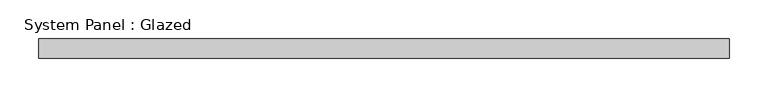
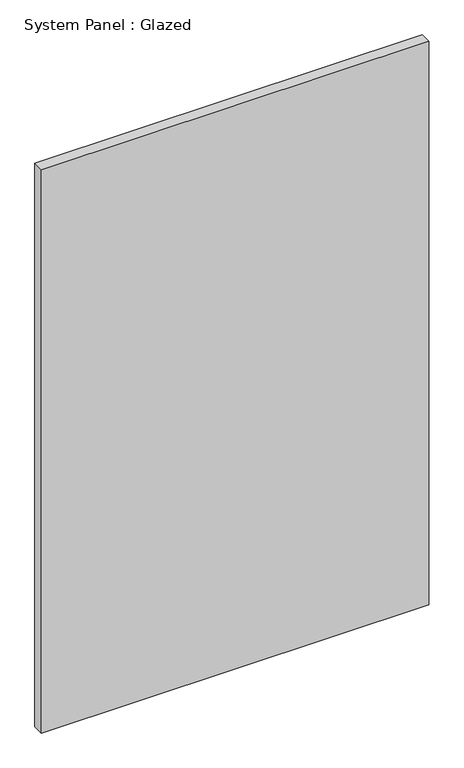
"""IFC4 building model written with IfcOpenShell, lengths in millimetres: plate geometry, System Panel : Glazed."""

from ifc_helpers import new_model, si_unit, origin, origin_with_axes, place, context, project, spatial, polyline, outline, extrude, source, transform, mapped, element, save


def system_panel_glazed_1adc8ad2(model_context):
    return source(origin(), model_context, "Body", "SweptSolid", [
        extrude(outline(polyline([(447.675, 19.05), (-447.675, 19.05), (-447.675, 44.45), (447.675, 44.45), (447.675, 19.05)])), origin_with_axes(), (0.0, 0.0, 1.0), 1376.5884629),
    ])


if __name__ == "__main__":
    model = new_model("IFC4")
    model_context = context("Model", 3, world=origin())
    ifc_project = project(units=[si_unit("LENGTHUNIT", "METRE", prefix="MILLI")], contexts=[model_context])
    site = spatial("IfcSite", under=ifc_project)
    building = spatial("IfcBuilding", under=site)
    placement = place(None, origin())
    system_panel_glazed_shape = system_panel_glazed_1adc8ad2(model_context)
    element("IfcPlate", 1, ObjectType="System Panel : Glazed", at=placement, inside=building, context=model_context, shape_type="MappedRepresentation", body=[
        mapped(system_panel_glazed_shape, transform((0.0, 0.0, 0.0), x_axis=(1.0, 0.0, 0.0), y_axis=(0.0, 1.0, 0.0), z_axis=(0.0, 0.0, 1.0))),
    ])
    save(model, "model.ifc")

# Revit data of these elements
# Type "System Panel : Glazed"
#   Construction Type Id = "GSP4R"
#   Analytic Construction = "1/8 in Pilkington single glazing"
#   Visual Light Transmittance = 0.9
#   Solar Heat Gain Coefficient = 0.86
#   Heat Transfer Coefficient (U) = 1.18115 BTU/(h·ft²·°F)
#   Define Thermal Properties by = 1
# Element 1 (IfcPlate, "System Panel : Glazed")
#   Materials on its faces: "Glass"
# Materials
#   "Glass": class "Glass", colour RGB 0 128 192, transparency 0.75, Description = "Soda Lime Glass", Cost = 0
